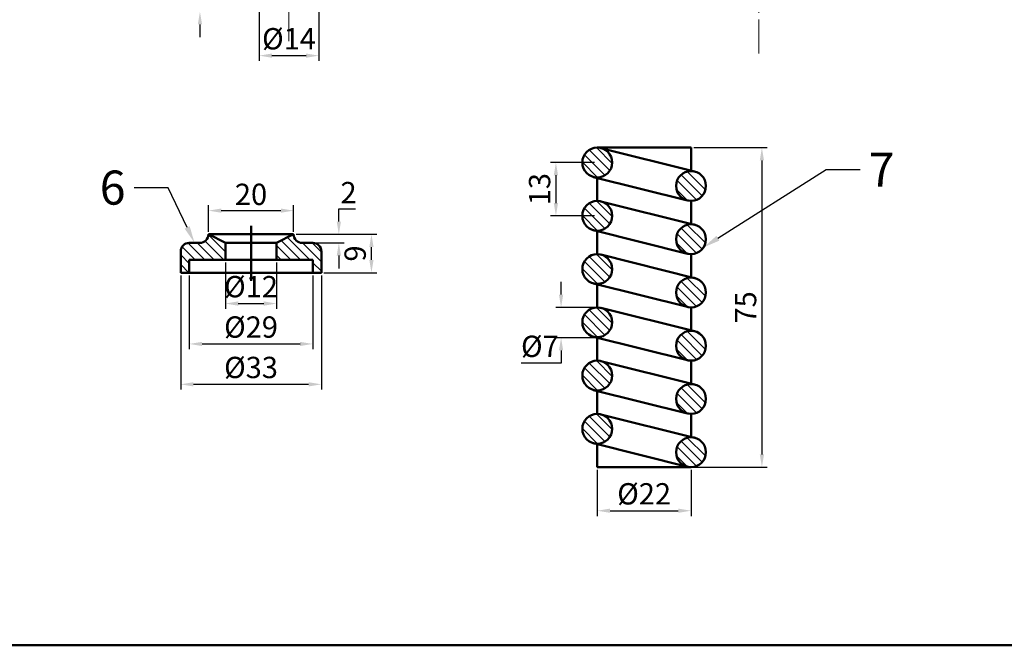
# Model space of a CAD drawing. Units: millimetres. Extents: x -656 to 85, y 134 to 571.
# Tile 2 of 5: x -409 to -178, y 134 to 281. Entities that reach past the tile are written whole.
import ezdxf
from ezdxf import colors
from ezdxf.entities.mleader import LeaderData, LeaderLine
from ezdxf.math import Vec2, Vec3

# ---------------------------------------------------------------- set-up
doc = ezdxf.new("R2010")
doc.units = ezdxf.units.MM
doc.header["$LTSCALE"] = 0.5
doc.linetypes.add('CENTER', pattern=[50.8, 31.75, -6.35, 6.35, -6.35])
for name, color, linetype, lineweight in [('M-CNTR', 1, 'CENTER', 18), ('M-DIMS', 2, 'Continuous', 25), ('M-HATC', 8, 'Continuous', 18), ('M-OUTL', 7, 'Continuous', 50), ('M-TEXT', 7, 'Continuous', 25), ('M-TTLB', 7, 'Continuous', 50)]:
    doc.layers.add(name, color=color, linetype=linetype, lineweight=lineweight)
doc.styles.get("Standard").update_dxf_attribs({"font": 'arial.ttf'})
doc.dimstyles.new('ISO-25', dxfattribs={"dimtxt": 5, "dimasz": 3, "dimexe": 1.25, "dimexo": 0.625, "dimtad": 1, "dimtoh": 1, "dimdec": 0, "dimtxsty": 'Standard', "dimcen": 2.5, "dimadec": 0, "dimazin": 0, "dimtfac": 1, "dimtdec": 0, "dimtofl": 0, "dimtmove": 0, "dimatfit": 3, "dimfxl": 1, "dimarcsym": 0})

# ---------------------------------------------------------------- blocks, each defined once
blk = doc.blocks.new('*D24')
at = {"layer": 'Defpoints', "color": 0, "ltscale": 0.5, "transparency": 16777216}
for p in [(-344.62, 236.52), (-364.62, 230.96), (-344.62, 230.96)]:
    blk.add_point(p, dxfattribs=at)
at = {"layer": 'M-DIMS', "color": 0, "lineweight": -2, "ltscale": 0.5, "transparency": 16777216}
for p, q in [((-364.62, 231.58), (-364.62, 237.77)), ((-361.62, 236.52), (-347.62, 236.52)), ((-344.62, 231.58), (-344.62, 237.77))]:
    blk.add_line(p, q, dxfattribs=at)
at = {"layer": 'M-DIMS', "color": 0, "ltscale": 0.5, "transparency": 16777216}
for points in [[(-361.62, 237.02), (-361.62, 236.02), (-364.62, 236.52)], [(-347.62, 237.02), (-347.62, 236.02), (-344.62, 236.52)]]:
    blk.add_solid(points, dxfattribs=at)
at = {"layer": 'M-DIMS', "color": 0, "ltscale": 0.5, "transparency": 16777216, "insert": (-354.62, 239.7), "char_height": 5, "attachment_point": 5}
blk.add_mtext('20', dxfattribs=at)
blk = doc.blocks.new('*D25')
at = {"layer": 'Defpoints', "color": 0, "ltscale": 0.5, "transparency": 16777216}
for p in [(-344.62, 230.96), (-342.62, 228.96), (-334.01, 228.96)]:
    blk.add_point(p, dxfattribs=at)
at = {"layer": 'M-DIMS', "color": 0, "lineweight": -2, "ltscale": 0.5, "transparency": 16777216}
for p, q in [((-334.01, 233.96), (-334.01, 236.96)), ((-334.01, 236.96), (-330.07, 236.96)), ((-344, 230.96), (-332.76, 230.96)), ((-342, 228.96), (-332.76, 228.96)), ((-334.01, 225.96), (-334.01, 222.96))]:
    blk.add_line(p, q, dxfattribs=at)
at = {"layer": 'M-DIMS', "color": 0, "ltscale": 0.5, "transparency": 16777216}
for points in [[(-334.51, 233.96), (-333.51, 233.96), (-334.01, 230.96)], [(-334.51, 225.96), (-333.51, 225.96), (-334.01, 228.96)]]:
    blk.add_solid(points, dxfattribs=at)
at = {"layer": 'M-DIMS', "color": 0, "ltscale": 0.5, "transparency": 16777216, "insert": (-331.73, 240.1), "char_height": 5, "attachment_point": 5}
blk.add_mtext('2', dxfattribs=at)
blk = doc.blocks.new('*D26')
at = {"layer": 'Defpoints', "color": 0, "ltscale": 0.5, "transparency": 16777216}
for p in [(-344.62, 230.96), (-326.36, 230.96), (-338.12, 221.96)]:
    blk.add_point(p, dxfattribs=at)
at = {"layer": 'M-DIMS', "color": 0, "lineweight": -2, "ltscale": 0.5, "transparency": 16777216}
for p, q in [((-344, 230.96), (-325.11, 230.96)), ((-326.36, 224.96), (-326.36, 227.96)), ((-337.5, 221.96), (-325.11, 221.96))]:
    blk.add_line(p, q, dxfattribs=at)
at = {"layer": 'M-DIMS', "color": 0, "ltscale": 0.5, "transparency": 16777216}
for points in [[(-326.86, 227.96), (-325.86, 227.96), (-326.36, 230.96)], [(-326.86, 224.96), (-325.86, 224.96), (-326.36, 221.96)]]:
    blk.add_solid(points, dxfattribs=at)
at = {"layer": 'M-DIMS', "color": 0, "ltscale": 0.5, "transparency": 16777216, "insert": (-329.54, 226.46), "char_height": 5, "attachment_point": 5, "rotation": 90}
blk.add_mtext('9', dxfattribs=at)
blk = doc.blocks.new('*D27')
at = {"layer": 'Defpoints', "color": 0, "ltscale": 0.5, "transparency": 16777216}
for p in [(-369.12, 221.96), (-340.12, 221.96), (-340.12, 205.23)]:
    blk.add_point(p, dxfattribs=at)
at = {"layer": 'M-DIMS', "color": 0, "lineweight": -2, "ltscale": 0.5, "transparency": 16777216}
for p, q in [((-369.12, 221.33), (-369.12, 203.98)), ((-340.12, 221.33), (-340.12, 203.98)), ((-366.12, 205.23), (-343.12, 205.23))]:
    blk.add_line(p, q, dxfattribs=at)
at = {"layer": 'M-DIMS', "color": 0, "ltscale": 0.5, "transparency": 16777216}
for points in [[(-366.12, 205.73), (-366.12, 204.73), (-369.12, 205.23)], [(-343.12, 205.73), (-343.12, 204.73), (-340.12, 205.23)]]:
    blk.add_solid(points, dxfattribs=at)
at = {"layer": 'M-DIMS', "color": 0, "ltscale": 0.5, "transparency": 16777216, "insert": (-354.62, 208.55), "char_height": 5, "attachment_point": 5}
blk.add_mtext('%%C29', dxfattribs=at)
blk = doc.blocks.new('*D28')
at = {"layer": 'Defpoints', "color": 0, "ltscale": 0.5, "transparency": 16777216}
for p in [(-371.12, 221.96), (-338.12, 221.96), (-338.12, 195.75)]:
    blk.add_point(p, dxfattribs=at)
at = {"layer": 'M-DIMS', "color": 0, "lineweight": -2, "ltscale": 0.5, "transparency": 16777216}
for p, q in [((-371.12, 221.33), (-371.12, 194.5)), ((-338.12, 221.33), (-338.12, 194.5)), ((-368.12, 195.75), (-341.12, 195.75))]:
    blk.add_line(p, q, dxfattribs=at)
at = {"layer": 'M-DIMS', "color": 0, "ltscale": 0.5, "transparency": 16777216}
for points in [[(-368.12, 196.25), (-368.12, 195.25), (-371.12, 195.75)], [(-341.12, 196.25), (-341.12, 195.25), (-338.12, 195.75)]]:
    blk.add_solid(points, dxfattribs=at)
at = {"layer": 'M-DIMS', "color": 0, "ltscale": 0.5, "transparency": 16777216, "insert": (-354.62, 199.06), "char_height": 5, "attachment_point": 5}
blk.add_mtext('%%C33', dxfattribs=at)
blk = doc.blocks.new('*D29')
at = {"layer": 'Defpoints', "color": 0, "ltscale": 0.5, "transparency": 16777216}
for p in [(-360.62, 224.96), (-348.62, 224.96), (-348.62, 214.71)]:
    blk.add_point(p, dxfattribs=at)
at = {"layer": 'M-DIMS', "color": 0, "lineweight": -2, "ltscale": 0.5, "transparency": 16777216}
for p, q in [((-360.62, 224.33), (-360.62, 213.46)), ((-348.62, 224.33), (-348.62, 213.46)), ((-357.62, 214.71), (-351.62, 214.71))]:
    blk.add_line(p, q, dxfattribs=at)
at = {"layer": 'M-DIMS', "color": 0, "ltscale": 0.5, "transparency": 16777216}
for points in [[(-357.62, 215.21), (-357.62, 214.21), (-360.62, 214.71)], [(-351.62, 215.21), (-351.62, 214.21), (-348.62, 214.71)]]:
    blk.add_solid(points, dxfattribs=at)
at = {"layer": 'M-DIMS', "color": 0, "ltscale": 0.5, "transparency": 16777216, "insert": (-354.62, 218.03), "char_height": 5, "attachment_point": 5}
blk.add_mtext('%%C12', dxfattribs=at)
blk = doc.blocks.new('*U56')
at = {"layer": 'M-CNTR', "color": 0, "transparency": 16777216}
blk.add_line((0, 51), (0, -85.46), dxfattribs=at)
blk = doc.blocks.new('*D62')
at = {"layer": 'Defpoints', "color": 0, "ltscale": 0.5, "transparency": 16777216}
for p in [(-352.71, 290.24), (-366.6, 283.24), (-345.71, 283.24)]:
    blk.add_point(p, dxfattribs=at)
at = {"layer": 'M-DIMS', "color": 0, "lineweight": -2, "ltscale": 0.5, "transparency": 16777216}
for p, q in [((-366.6, 293.24), (-366.6, 296.24)), ((-353.33, 290.24), (-367.85, 290.24)), ((-346.33, 283.24), (-367.85, 283.24)), ((-366.6, 280.24), (-366.6, 277.24))]:
    blk.add_line(p, q, dxfattribs=at)
at = {"layer": 'M-DIMS', "color": 0, "ltscale": 0.5, "transparency": 16777216}
for points in [[(-367.1, 293.24), (-366.1, 293.24), (-366.6, 290.24)], [(-367.1, 280.24), (-366.1, 280.24), (-366.6, 283.24)]]:
    blk.add_solid(points, dxfattribs=at)
at = {"layer": 'M-DIMS', "color": 0, "ltscale": 0.5, "transparency": 16777216, "insert": (-369.73, 286.74), "char_height": 5, "attachment_point": 5, "rotation": 90}
blk.add_mtext('7', dxfattribs=at)
blk = doc.blocks.new('*D66')
at = {"layer": 'Defpoints', "color": 0, "ltscale": 0.5, "transparency": 16777216}
for p in [(-352.71, 290.24), (-338.71, 290.24), (-338.71, 272.9)]:
    blk.add_point(p, dxfattribs=at)
at = {"layer": 'M-DIMS', "color": 0, "lineweight": -2, "ltscale": 0.5, "transparency": 16777216}
for p, q in [((-352.71, 289.61), (-352.71, 271.65)), ((-338.71, 289.61), (-338.71, 271.65)), ((-349.71, 272.9), (-341.71, 272.9))]:
    blk.add_line(p, q, dxfattribs=at)
at = {"layer": 'M-DIMS', "color": 0, "ltscale": 0.5, "transparency": 16777216}
for points in [[(-349.71, 273.4), (-349.71, 272.4), (-352.71, 272.9)], [(-341.71, 273.4), (-341.71, 272.4), (-338.71, 272.9)]]:
    blk.add_solid(points, dxfattribs=at)
at = {"layer": 'M-DIMS', "color": 0, "ltscale": 0.5, "transparency": 16777216, "insert": (-345.71, 276.22), "char_height": 5, "attachment_point": 5}
blk.add_mtext('%%C14', dxfattribs=at)
blk = doc.blocks.new('*D74')
at = {"layer": 'Defpoints', "color": 0, "ltscale": 0.5, "transparency": 16777216}
for p in [(-273.38, 247.81), (-283.08, 235.31), (-273.38, 235.31)]:
    blk.add_point(p, dxfattribs=at)
at = {"layer": 'M-DIMS', "color": 0, "lineweight": -2, "ltscale": 0.5, "transparency": 16777216}
for p, q in [((-274.01, 247.81), (-284.33, 247.81)), ((-283.08, 244.81), (-283.08, 238.31)), ((-274.01, 235.31), (-284.33, 235.31))]:
    blk.add_line(p, q, dxfattribs=at)
at = {"layer": 'M-DIMS', "color": 0, "ltscale": 0.5, "transparency": 16777216}
for points in [[(-283.58, 244.81), (-282.58, 244.81), (-283.08, 247.81)], [(-283.58, 238.31), (-282.58, 238.31), (-283.08, 235.31)]]:
    blk.add_solid(points, dxfattribs=at)
at = {"layer": 'M-DIMS', "color": 0, "ltscale": 0.5, "transparency": 16777216, "insert": (-286.26, 241.56), "char_height": 5, "attachment_point": 5, "rotation": 90}
blk.add_mtext('13', dxfattribs=at)
blk = doc.blocks.new('*D75')
at = {"layer": 'Defpoints', "color": 0, "ltscale": 0.5, "transparency": 16777216}
for p in [(-251.38, 251.31), (-251.38, 176.31), (-234.75, 176.31)]:
    blk.add_point(p, dxfattribs=at)
at = {"layer": 'M-DIMS', "color": 0, "lineweight": -2, "ltscale": 0.5, "transparency": 16777216}
for p, q in [((-250.76, 251.31), (-233.5, 251.31)), ((-234.75, 248.31), (-234.75, 179.31)), ((-250.76, 176.31), (-233.5, 176.31))]:
    blk.add_line(p, q, dxfattribs=at)
at = {"layer": 'M-DIMS', "color": 0, "ltscale": 0.5, "transparency": 16777216}
for points in [[(-235.25, 248.31), (-234.25, 248.31), (-234.75, 251.31)], [(-235.25, 179.31), (-234.25, 179.31), (-234.75, 176.31)]]:
    blk.add_solid(points, dxfattribs=at)
at = {"layer": 'M-DIMS', "color": 0, "ltscale": 0.5, "transparency": 16777216, "insert": (-237.92, 213.81), "char_height": 5, "attachment_point": 5, "rotation": 90}
blk.add_mtext('75', dxfattribs=at)
blk = doc.blocks.new('*D76')
at = {"layer": 'Defpoints', "color": 0, "ltscale": 0.5, "transparency": 16777216}
for p in [(-273.38, 176.31), (-251.38, 176.31), (-251.38, 166.08)]:
    blk.add_point(p, dxfattribs=at)
at = {"layer": 'M-DIMS', "color": 0, "lineweight": -2, "ltscale": 0.5, "transparency": 16777216}
for p, q in [((-273.38, 175.68), (-273.38, 164.83)), ((-251.38, 175.68), (-251.38, 164.83)), ((-270.38, 166.08), (-254.38, 166.08))]:
    blk.add_line(p, q, dxfattribs=at)
at = {"layer": 'M-DIMS', "color": 0, "ltscale": 0.5, "transparency": 16777216}
for points in [[(-270.38, 166.58), (-270.38, 165.58), (-273.38, 166.08)], [(-254.38, 166.58), (-254.38, 165.58), (-251.38, 166.08)]]:
    blk.add_solid(points, dxfattribs=at)
at = {"layer": 'M-DIMS', "color": 0, "ltscale": 0.5, "transparency": 16777216, "insert": (-262.38, 169.4), "char_height": 5, "attachment_point": 5}
blk.add_mtext('%%C22', dxfattribs=at)
blk = doc.blocks.new('*D77')
at = {"layer": 'Defpoints', "color": 0, "ltscale": 0.5, "transparency": 16777216}
for p in [(-273.38, 213.81), (-281.87, 206.7), (-273.38, 206.7)]:
    blk.add_point(p, dxfattribs=at)
at = {"layer": 'M-DIMS', "color": 0, "lineweight": -2, "ltscale": 0.5, "transparency": 16777216}
for p, q in [((-281.87, 216.81), (-281.87, 219.81)), ((-274.01, 213.81), (-283.12, 213.81)), ((-274.01, 206.7), (-283.12, 206.7)), ((-281.87, 203.7), (-281.87, 200.7)), ((-281.87, 200.7), (-291.21, 200.7))]:
    blk.add_line(p, q, dxfattribs=at)
at = {"layer": 'M-DIMS', "color": 0, "ltscale": 0.5, "transparency": 16777216}
for points in [[(-282.37, 216.81), (-281.37, 216.81), (-281.87, 213.81)], [(-282.37, 203.7), (-281.37, 203.7), (-281.87, 206.7)]]:
    blk.add_solid(points, dxfattribs=at)
at = {"layer": 'M-DIMS', "color": 0, "ltscale": 0.5, "transparency": 16777216, "insert": (-286.85, 204.02), "char_height": 5, "attachment_point": 5}
blk.add_mtext('%%C7', dxfattribs=at)

msp = doc.modelspace()

# ---------------------------------------------------------------- hatches: boundary and pattern name
at = {"layer": 'M-HATC', "ltscale": 0.5}
h = msp.add_hatch(dxfattribs=at)
h.set_pattern_fill('ANSI31', color=256, scale=0.5, angle=90)
h.set_pattern_definition([(135, (-1755.2787, -76.5175), (-1.122532, -1.122532), [])])
h.paths.add_polyline_path([(-276.88, 247.81, 1), (-269.88, 247.81, 1)])
h.paths.add_polyline_path([(-254.88, 242.31, 1), (-247.88, 242.31, 1)])
h = msp.add_hatch(dxfattribs=at)
h.set_pattern_fill('ANSI31', color=256, scale=0.5, angle=90)
h.set_pattern_definition([(135, (-1755.2787, -89.0175), (-1.122532, -1.122532), [])])
h.paths.add_polyline_path([(-276.88, 235.31, 1), (-269.88, 235.31, 1)])
h.paths.add_polyline_path([(-254.88, 229.81, 1), (-247.88, 229.81, 1)])
h = msp.add_hatch(dxfattribs=at)
h.set_pattern_fill('ANSI31', color=256, scale=0.5, angle=90)
h.set_pattern_definition([(135, (-1588.6692, -80.7438), (-1.122532, -1.122532), [])])
h.paths.add_polyline_path([(-360.62, 224.96), (-360.62, 228.96), (-364.62, 230.96, -0.414214), (-366.62, 228.96), (-369.12, 228.96, 0.414214), (-371.12, 226.96), (-371.12, 221.96), (-369.12, 221.96), (-369.12, 224.96)])
h.paths.add_polyline_path([(-340.12, 224.96), (-340.12, 221.96), (-338.12, 221.96), (-338.12, 226.96, 0.414214), (-340.12, 228.96), (-342.62, 228.96, -0.414214), (-344.62, 230.96), (-348.62, 228.96), (-348.62, 224.96)])
h = msp.add_hatch(dxfattribs=at)
h.set_pattern_fill('ANSI31', color=256, scale=0.5, angle=90)
h.set_pattern_definition([(135, (-1755.2787, -101.5175), (-1.122532, -1.122532), [])])
h.paths.add_polyline_path([(-276.88, 222.81, 1), (-269.88, 222.81, 1)])
h.paths.add_polyline_path([(-254.88, 217.31, 1), (-247.88, 217.31, 1)])
h = msp.add_hatch(dxfattribs=at)
h.set_pattern_fill('ANSI31', color=256, scale=0.5, angle=90)
h.set_pattern_definition([(135, (-1755.2787, -114.0175), (-1.122532, -1.122532), [])])
h.paths.add_polyline_path([(-276.88, 210.31, 1), (-269.88, 210.31, 1)])
h.paths.add_polyline_path([(-254.88, 204.81, 1), (-247.88, 204.81, 1)])
h = msp.add_hatch(dxfattribs=at)
h.set_pattern_fill('ANSI31', color=256, scale=0.5, angle=90)
h.set_pattern_definition([(135, (-1755.2787, -126.5175), (-1.122532, -1.122532), [])])
h.paths.add_polyline_path([(-276.88, 197.81, 1), (-269.88, 197.81, 1)])
h.paths.add_polyline_path([(-254.88, 192.31, 1), (-247.88, 192.31, 1)])
h = msp.add_hatch(dxfattribs=at)
h.set_pattern_fill('ANSI31', color=256, scale=0.5, angle=90)
h.set_pattern_definition([(135, (-1755.2787, -139.0175), (-1.122532, -1.122532), [])])
h.paths.add_polyline_path([(-276.88, 185.31, 1), (-269.88, 185.31, 1)])
h.paths.add_polyline_path([(-254.88, 179.81, 1), (-247.88, 179.81, 1)])

# ---------------------------------------------------------------- linework, layer by layer
at = {"layer": 'M-CNTR', "ltscale": 0.5}
msp.add_line((-235.5, 273.42), (-235.5, 341.1), dxfattribs=at)
at = {"layer": 'M-OUTL', "ltscale": 0.5}
for p, q in [((-251.38, 251.31), (-273.38, 251.31)), ((-272.54, 251.2), (-250.54, 245.7)), ((-251.38, 251.31), (-251.38, 245.81)), ((-251.38, 245.81), (-251.38, 251.31)), ((-274.23, 244.41), (-252.23, 238.91)), ((-273.38, 244.31), (-273.38, 238.81)), ((-272.54, 238.7), (-250.54, 233.2)), ((-251.38, 233.31), (-251.38, 238.81)), ((-354.62, 220.03), (-354.62, 232.96)), ((-274.23, 231.91), (-252.23, 226.41)), ((-273.38, 231.81), (-273.38, 226.31)), ((-369.12, 228.96), (-366.62, 228.96)), ((-364.62, 230.96), (-344.62, 230.96)), ((-364.62, 230.96), (-344.62, 230.96)), ((-360.62, 228.96), (-364.62, 230.96)), ((-360.62, 224.96), (-360.62, 228.96)), ((-360.62, 228.96), (-348.62, 228.96)), ((-348.62, 228.96), (-344.62, 230.96)), ((-348.62, 224.96), (-348.62, 228.96)), ((-342.62, 228.96), (-340.12, 228.96)), ((-371.12, 226.96), (-371.12, 221.96)), ((-338.12, 221.96), (-338.12, 226.96)), ((-369.12, 224.96), (-340.12, 224.96)), ((-369.12, 224.96), (-369.12, 221.96)), ((-369.12, 224.96), (-340.12, 224.96)), ((-340.12, 224.96), (-340.12, 221.96)), ((-272.54, 226.2), (-250.54, 220.7)), ((-251.38, 220.81), (-251.38, 226.31)), ((-371.12, 221.96), (-338.12, 221.96)), ((-274.23, 219.41), (-252.23, 213.91)), ((-273.38, 219.31), (-273.38, 213.81)), ((-272.54, 213.7), (-250.54, 208.2)), ((-251.38, 208.31), (-251.38, 213.81)), ((-274.23, 206.91), (-252.23, 201.41)), ((-273.38, 206.81), (-273.38, 201.31)), ((-272.54, 201.2), (-250.54, 195.7)), ((-251.38, 195.81), (-251.38, 201.31)), ((-274.23, 194.41), (-252.23, 188.91)), ((-273.38, 194.31), (-273.38, 188.81)), ((-272.54, 188.7), (-250.54, 183.2)), ((-251.38, 183.31), (-251.38, 188.81)), ((-274.23, 181.91), (-252.23, 176.41)), ((-273.38, 181.81), (-273.38, 176.31)), ((-273.38, 176.31), (-251.38, 176.31))]:
    msp.add_line(p, q, dxfattribs=at)
for centre in [(-273.38, 247.81), (-251.38, 242.31), (-273.38, 235.31), (-251.38, 229.81), (-273.38, 222.81), (-251.38, 217.31), (-273.38, 210.31), (-251.38, 204.81), (-273.38, 197.81), (-251.38, 192.31), (-273.38, 185.31), (-251.38, 179.81)]:
    msp.add_circle(centre, 3.5, dxfattribs=at)
for centre, start, end in [((-369.12, 226.96), 90, 180), ((-366.62, 230.96), 270, 0), ((-342.62, 230.96), 180, 270), ((-340.12, 226.96), 0, 90)]:
    msp.add_arc(centre, 2, start, end, dxfattribs=at)
at = {"layer": 'M-TTLB', "ltscale": 0.5}
msp.add_lwpolyline([(-656.34, 571.01), (84.63, 571.01), (84.63, 134.49), (-656.34, 134.49)], close=True, dxfattribs=at)

# ---------------------------------------------------------------- block references
at = {"layer": 'M-CNTR'}
msp.add_blockref('*U56', (-345.71, 361.74), dxfattribs=at)

# ---------------------------------------------------------------- dimensions: what is measured, and where the dimension line sits
at = {"layer": 'M-DIMS', "ltscale": 0.5}
for base, p1, p2, picture, middle in [((-366.6, 283.24), (-352.71, 290.24), (-345.71, 283.24), '*D62', (-369.73, 286.74)), ((-234.75, 176.31), (-251.38, 251.31), (-251.38, 176.31), '*D75', (-237.92, 213.81)), ((-283.08099647, 235.30559333), (-273.38418342, 247.80559333), (-273.38418342, 235.30559333), '*D74', (-286.26056673, 241.55559333)), ((-326.36, 230.96), (-338.12, 221.96), (-344.62, 230.96), '*D26', (-329.54, 226.46))]:
    dim = msp.add_linear_dim(base=base, p1=p1, p2=p2, angle=90, dimstyle='ISO-25', override={"dimclrd": 0, "dimclre": 0, "dimclrt": 0}, dxfattribs=at)
    dim.commit()
    dim.dimension.update_dxf_attribs({"geometry": picture, "text_midpoint": middle})
for base, p1, p2, picture, middle in [((-338.71, 272.9), (-352.71, 290.24), (-338.71, 290.24), '*D66', (-345.71, 276.22)), ((-251.38, 166.08), (-273.38, 176.31), (-251.38, 176.31), '*D76', (-262.38, 169.4))]:
    dim = msp.add_linear_dim(base=base, p1=p1, p2=p2, text='%%C<>', dimstyle='ISO-25', override={"dimclrd": 0, "dimclre": 0, "dimclrt": 0}, dxfattribs=at)
    dim.commit()
    dim.dimension.update_dxf_attribs({"geometry": picture, "text_midpoint": middle})
dim = msp.add_linear_dim(base=(-344.62, 236.52), p1=(-364.62, 230.96), p2=(-344.62, 230.96), dimstyle='ISO-25', override={"dimclrd": 0, "dimclre": 0, "dimclrt": 0}, dxfattribs=at)
dim.commit()
dim.dimension.update_dxf_attribs({"geometry": '*D24', "text_midpoint": (-354.62, 239.7)})
dim = msp.add_linear_dim(base=(-334.01, 228.96), p1=(-344.62, 230.96), p2=(-342.62, 228.96), angle=90, dimstyle='ISO-25', override={"dimclrd": 0, "dimclre": 0, "dimclrt": 0}, dxfattribs=at)
dim.commit()
dim.dimension.update_dxf_attribs({"geometry": '*D25', "text_midpoint": (-331.73, 236.96), "dimtype": 160})
for base, p1, p2, picture, middle in [((-348.62, 214.71), (-360.62, 224.96), (-348.62, 224.96), '*D29', (-354.62, 214.71)), ((-338.12, 195.75), (-371.12, 221.96), (-338.12, 221.96), '*D28', (-354.62, 195.75)), ((-340.12, 205.23), (-369.12, 221.96), (-340.12, 221.96), '*D27', (-354.62, 205.23))]:
    dim = msp.add_linear_dim(base=base, p1=p1, p2=p2, text='%%C<>', dimstyle='ISO-25', override={"dimclrd": 0, "dimclre": 0, "dimclrt": 0}, dxfattribs=at)
    dim.commit()
    dim.dimension.update_dxf_attribs({"geometry": picture, "text_midpoint": middle, "dimtype": 160})
dim = msp.add_linear_dim(base=(-281.87, 206.7), p1=(-273.38, 213.81), p2=(-273.38, 206.7), angle=90, text='%%C<>', dimstyle='ISO-25', override={"dimclrd": 0, "dimclre": 0, "dimclrt": 0}, dxfattribs=at)
dim.commit()
dim.dimension.update_dxf_attribs({"geometry": '*D77', "text_midpoint": (-286.85, 204.02)})

# ---------------------------------------------------------------- leaders
at = {"layer": 'M-TEXT', "ltscale": 0.5}
ml = msp.add_multileader_mtext('Standard', dxfattribs=at)
ml.set_content('7', color=256)
ml.set_leader_properties()
ml.build(insert=Vec2(0, 0))
ctx = ml.context
ctx.base_point, ctx.char_height, ctx.plane_origin = Vec3(-211.69, 246.15), 8, Vec3(-248.46, 227.89)
notes = []
notes.append((ctx, [(0, (1, 1, 0), (-219.69, 246.15), (1, 0), 8, [(0, [(-248.46, 227.89)], 0, [])])]))
ctx.mtext.insert, ctx.mtext.flow_direction = Vec3(-209.69, 250.15), 5
ml = msp.add_multileader_mtext('Standard', dxfattribs=at)
ml.set_content('6', color=256)
ml.set_leader_properties()
ml.build(insert=Vec2(0, 0))
ctx = ml.context
ctx.base_point, ctx.char_height, ctx.plane_origin = Vec3(-391.34, 241.86), 8, Vec3(-367.87, 228.96)
ctx.text_align_type = 2
notes.append((ctx, [(0, (1, 1, 0), (-374.06, 241.86), (-1, 0), 8, [(0, [(-367.87, 228.96)], 0, [])])]))
ctx.mtext.insert, ctx.mtext.alignment, ctx.mtext.flow_direction = Vec3(-384.06, 245.93), 3, 5
for ctx, leaders in notes:
    for number, flags, end, landing, length, lines in leaders:
        leader = LeaderData()
        leader.index, (leader.has_last_leader_line, leader.has_dogleg_vector, leader.attachment_direction) = number, flags
        leader.last_leader_point, leader.dogleg_vector, leader.dogleg_length = Vec3(end), Vec3(landing), length
        for number, points, colour, breaks in lines:
            line = LeaderLine()
            line.index, line.vertices, line.color, line.breaks = number, Vec3.list(points), colors.encode_raw_color(colour), breaks
            leader.lines.append(line)
        ctx.leaders.append(leader)

doc.saveas('drawing.dxf')
